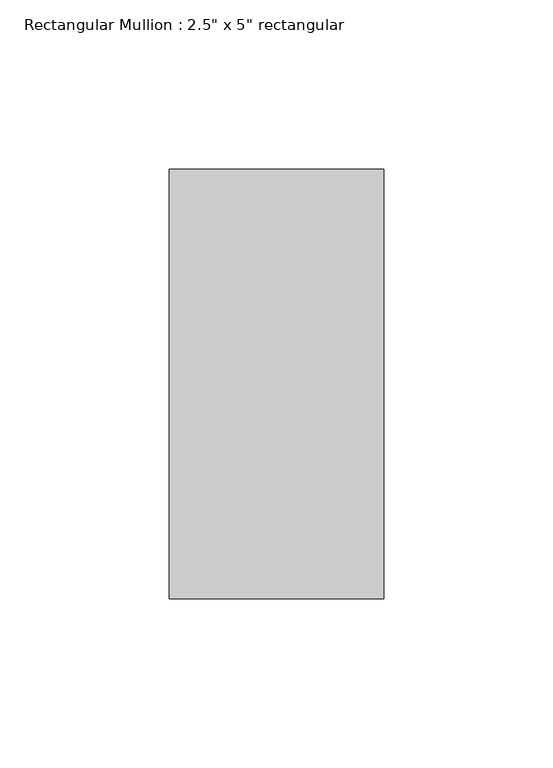
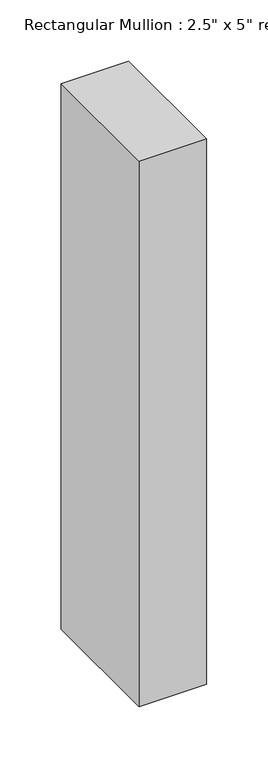
"""IFC4 building model written with IfcOpenShell, lengths in millimetres: member geometry."""

from ifc_helpers import new_model, si_unit, frame, origin, place, context, project, spatial, polyline, outline, extrude, source, transform, mapped, element, save


def member_eeaa8261(model_context):
    return source(origin(), model_context, "Body", "SweptSolid", [
        extrude(outline(polyline([(31.75, 63.5), (31.75, -63.5), (-31.75, -63.5), (-31.75, 63.5), (31.75, 63.5)])), frame((0.0, 0.0, -542.1748327), z_axis=(0.0, 0.0, 1.0), x_axis=(1.0, 0.0, 0.0)), (0.0, 0.0, 1.0), 542.1748327),
    ])


if __name__ == "__main__":
    model = new_model("IFC4")
    model_context = context("Model", 3, world=origin())
    ifc_project = project(units=[si_unit("LENGTHUNIT", "METRE", prefix="MILLI")], contexts=[model_context])
    site = spatial("IfcSite", under=ifc_project)
    building = spatial("IfcBuilding", under=site)
    placement = place(None, origin())
    member_shape = member_eeaa8261(model_context)
    element("IfcMember", 1, ObjectType="Rectangular Mullion : 2.5\" x 5\" rectangular", at=placement, inside=building, context=model_context, shape_type="MappedRepresentation", body=[
        mapped(member_shape, transform((0.0, 0.0, 0.0), x_axis=(1.0, 0.0, 0.0), y_axis=(0.0, 1.0, 0.0), z_axis=(0.0, 0.0, 1.0))),
    ])
    save(model, "model.ifc")

# Revit data of these elements
# Type "Rectangular Mullion : 2.5\" x 5\" rectangular"
#   built-in parameter 1007304 = 0.416667 (stored number, unit not read)
#   built-in parameter 1007301 = 0.104167 (stored number, unit not read)
#   built-in parameter 1007300 = 0.104167 (stored number, unit not read)
# Element 1 (IfcMember, "Rectangular Mullion : 2.5\" x 5\" rectangular")
#   Materials on its faces: "Aluminum"
# Materials
#   "Aluminum": class "Metal", colour RGB 247 247 247, transparency 0, Description = "Aluminum 6061", Cost = 0
